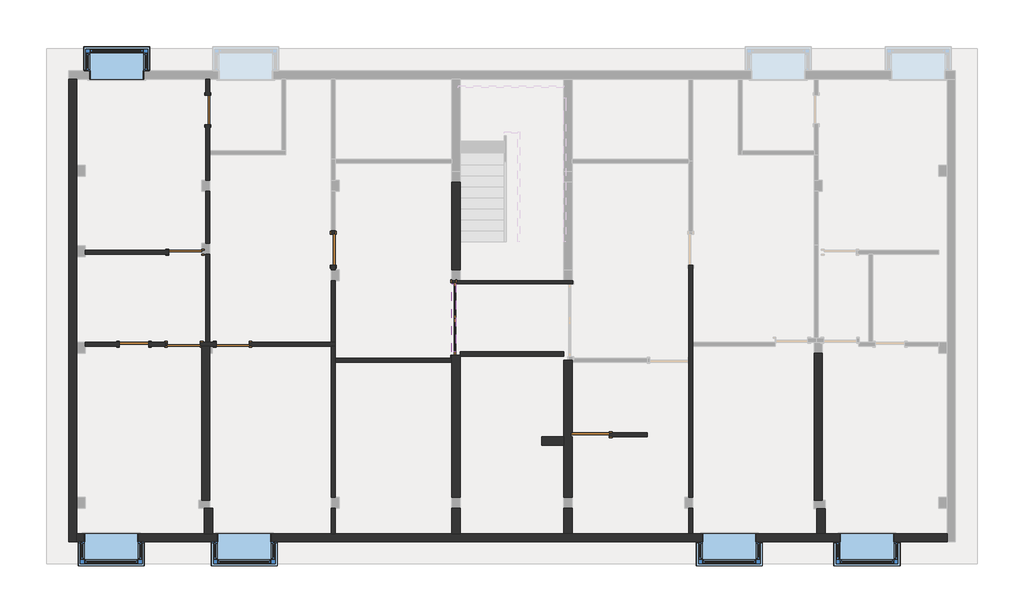
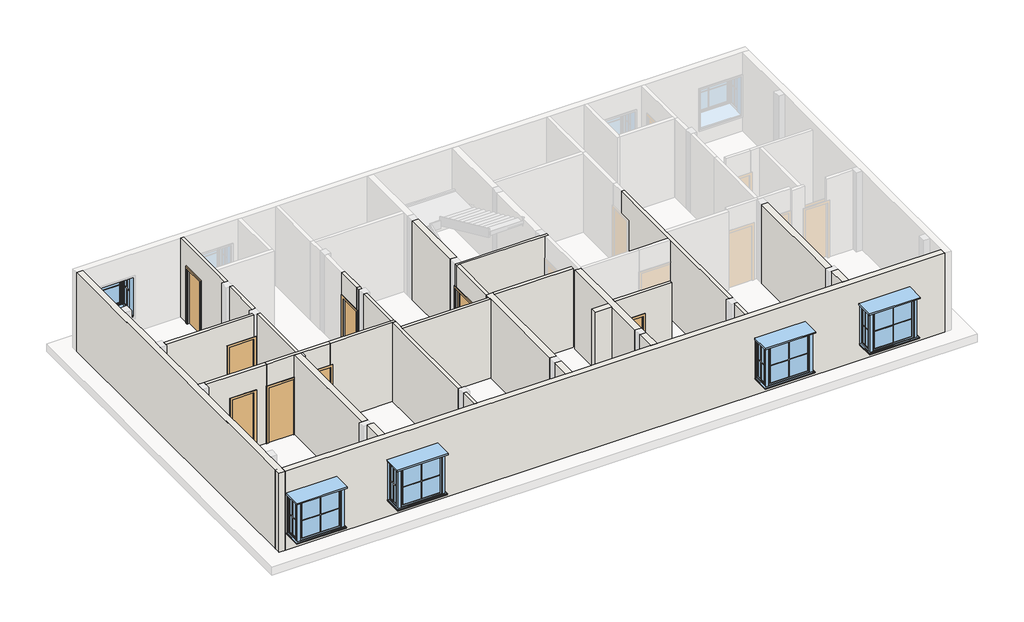
# One storey, part 1 of 3: 32 walls, 8 doors, 5 windows.
"""IFC4 building model written with IfcOpenShell, lengths in millimetres."""

from ifc_helpers import new_model, si_unit, frame, origin, place, context, project, spatial, polyline, outline, extrude, faceted_brep, transform, mapped, element, save
from components import door_04ab2522, m_door_single_panel_05506f71, door_07b5d71c, door_4c0a2014, door_82def9da, m_door_single_panel_3_x7_f8176753, m_door_single_panel_3_x7_ebb67e73, window_19bbd869

model = new_model("IFC4")

# Units and contexts
model_context = context("Model", 3, world=origin())
ifc_project = project(units=[si_unit("LENGTHUNIT", "METRE", prefix="MILLI")], contexts=[model_context])

# Site, building, storey
site = spatial("IfcSite", under=ifc_project)
building = spatial("IfcBuilding", under=site)
storey = spatial("IfcBuildingStorey", under=building, Elevation=6400.8)

# Doors
placement = place(None, origin())
door_shape = door_04ab2522(model_context)
element("IfcDoor", 1, ObjectType="M_Door-Double-Glass : 6'7\"X7'", at=placement, inside=storey, context=model_context, shape_type="MappedRepresentation", body=[
    mapped(door_shape, transform((-2022.6300498, 1231.0067742, 6400.8), x_axis=(0.0, -1.0, 0.0), y_axis=(1.0, 0.0, 0.0), z_axis=(0.0, 0.0, 1.0))),
])
m_door_single_panel_shape = m_door_single_panel_05506f71(model_context)
element("IfcDoor", 2, ObjectType="M_Door-Single-Panel", at=placement, inside=storey, context=model_context, shape_type="MappedRepresentation", body=[
    mapped(m_door_single_panel_shape, transform((1745.3012085, -1975.7432663, 6400.8), x_axis=(-1.0, 0.0, 0.0), y_axis=(0.0, -1.0, 0.0), z_axis=(0.0, 0.0, 1.0))),
])
door_2_shape = door_07b5d71c(model_context)
element("IfcDoor", 3, ObjectType="M_Door-Single-Panel : 2'10\"X7' 2", at=placement, inside=storey, context=model_context, shape_type="MappedRepresentation", body=[
    mapped(door_2_shape, transform((-5360.3487995, 3142.9626891, 6400.8), x_axis=(0.0, -1.0, 0.0), y_axis=(1.0, 0.0, 0.0), z_axis=(0.0, 0.0, 1.0))),
])
door_3_shape = door_4c0a2014(model_context)
element("IfcDoor", 4, ObjectType="M_Door-Single-Panel : 2'8\"X7'", at=placement, inside=storey, context=model_context, shape_type="MappedRepresentation", body=[
    mapped(door_3_shape, transform((-10873.4462614, 526.1567334, 6400.8), x_axis=(1.0, 0.0, 0.0), y_axis=(0.0, 1.0, 0.0), z_axis=(0.0, 0.0, 1.0))),
])
door_4_shape = door_82def9da(model_context)
element("IfcDoor", 5, ObjectType="M_Door-Single-Panel : 2'8\"X7'", at=placement, inside=storey, context=model_context, shape_type="MappedRepresentation", body=[
    mapped(door_4_shape, transform((-8827.4487992, 7008.6751452, 6400.8), x_axis=(0.0, 1.0, 0.0), y_axis=(-1.0, 0.0, 0.0), z_axis=(0.0, 0.0, 1.0))),
])
m_door_single_panel_3_x7_shape = m_door_single_panel_3_x7_f8176753(model_context)
element("IfcDoor", 6, ObjectType="M_Door-Single-Panel : 3'X7'", at=placement, inside=storey, context=model_context, shape_type="MappedRepresentation", body=[
    mapped(m_door_single_panel_3_x7_shape, transform((-9456.0987989, 3078.8567332, 6400.8), x_axis=(1.0, 0.0, 0.0), y_axis=(0.0, 1.0, 0.0), z_axis=(0.0, 0.0, 1.0))),
])
element("IfcDoor", 7, ObjectType="M_Door-Single-Panel : 3'X7'", at=placement, inside=storey, context=model_context, shape_type="MappedRepresentation", body=[
    mapped(m_door_single_panel_3_x7_shape, transform((-8144.8381465, 526.1567334, 6400.8), x_axis=(-1.0, 0.0, 0.0), y_axis=(0.0, -1.0, 0.0), z_axis=(0.0, 0.0, 1.0))),
])
m_door_single_panel_3_x7_2_shape = m_door_single_panel_3_x7_ebb67e73(model_context)
element("IfcDoor", 8, ObjectType="M_Door-Single-Panel : 3'X7'", at=placement, inside=storey, context=model_context, shape_type="MappedRepresentation", body=[
    mapped(m_door_single_panel_3_x7_2_shape, transform((-9494.1987992, 526.1567334, 6400.8), x_axis=(1.0, 0.0, 0.0), y_axis=(0.0, 1.0, 0.0), z_axis=(0.0, 0.0, 1.0))),
])

# Walls
element("IfcWall", 9, ObjectType="3.5\"", at=placement, inside=storey, context=model_context, shape_type="Brep", body=[
    faceted_brep([(1272.3082462, 2196.2067742, 9448.8), (1158.0082462, 2196.2067742, 9448.8), (-1963.0987998, 2196.2067742, 9448.8), (-2077.3987998, 2196.2067742, 9448.8), (-2077.3987998, 2196.2067742, 8534.4), (-1963.0987998, 2196.2067742, 8534.4), (-1963.0987998, 2196.2067742, 6400.8), (1158.0082462, 2196.2067742, 6400.8), (1272.3082462, 2196.2067742, 6400.8), (1272.3082462, 2285.1067742, 6400.8), (1253.2582462, 2285.1067742, 6400.8), (1024.6582462, 2285.1067742, 6400.8), (-1845.5417538, 2285.1067742, 6400.8), (-2074.1417538, 2285.1067742, 6400.8), (-2077.3987998, 2285.1067742, 6400.8), (-2077.3987998, 2285.1067742, 9448.8), (-2074.1417538, 2285.1067742, 9448.8), (-1845.5417538, 2285.1067742, 9448.8), (1024.6582462, 2285.1067742, 9448.8), (1253.2582462, 2285.1067742, 9448.8), (1272.3082462, 2285.1067742, 9448.8), (-1963.0987998, 2234.3067742, 6400.8), (-2077.3987998, 2234.3067742, 6400.8), (-2077.3987998, 2234.3067742, 8534.4), (-1963.0987998, 2234.3067742, 8534.4)], [[[0, 1, 2, 3, 4, 5, 6, 7, 8]], [[9, 10, 11, 12, 13, 14, 15, 16, 17, 18, 19, 20]], [[14, 13, 12, 11, 10, 9, 8, 7, 6, 21, 22]], [[3, 2, 1, 0, 20, 19, 18, 17, 16, 15]], [[0, 8, 9, 20]], [[3, 15, 14, 22, 23, 4]], [[24, 21, 6, 5]], [[23, 24, 5, 4]], [[21, 24, 23, 22]]]),
])
element("IfcWall", 10, ObjectType="4.5\"", at=placement, inside=storey, context=model_context, shape_type="SweptSolid", body=[
    extrude(outline(polyline([(2711.1626891, 9448.8), (3671.8272228, 9448.8), (3671.8272228, 6400.8), (3574.7626891, 6400.8), (3574.7626891, 8534.4), (2711.1626891, 8534.4), (2711.1626891, 9448.8)])), frame((-5417.4987995, 0.0, 0.0), z_axis=(1.0, 0.0, 0.0), x_axis=(0.0, 1.0, 0.0)), (0.0, 0.0, 1.0), 114.3),
])
element("IfcWall", 11, ObjectType="4.5\"", at=placement, inside=storey, context=model_context, shape_type="Brep", body=[
    faceted_brep([(-7690.1644155, 469.0067334, 9448.8), (-8713.148796, 469.0067334, 9448.8), (-8771.750543, 469.0067334, 9448.8), (-9000.350543, 469.0067334, 9448.8), (-10009.8462614, 469.0067334, 9448.8), (-10009.8462614, 469.0067334, 6400.8), (-9951.3987992, 469.0067334, 6400.8), (-9951.3987992, 469.0067334, 8534.4), (-9036.9987992, 469.0067334, 8534.4), (-9036.9987992, 469.0067334, 6400.8), (-9000.350543, 469.0067334, 6400.8), (-8771.750543, 469.0067334, 6400.8), (-8713.148796, 469.0067334, 6400.8), (-8602.0381465, 469.0067334, 6400.8), (-8602.0381465, 469.0067334, 8534.4), (-7690.1644155, 469.0067334, 8534.4), (-10009.8462614, 583.3067334, 9448.8), (-7690.1644155, 583.3067334, 9448.8), (-7690.1644155, 583.3067334, 8534.4), (-8602.0381465, 583.3067334, 8534.4), (-8602.0381465, 583.3067334, 6400.8), (-9036.9987992, 583.3067334, 6400.8), (-9036.9987992, 583.3067334, 8534.4), (-9951.3987992, 583.3067334, 8534.4), (-9951.3987992, 583.3067334, 6400.8), (-10009.8462614, 583.3067334, 6400.8)], [[[0, 1, 2, 3, 4, 5, 6, 7, 8, 9, 10, 11, 12, 13, 14, 15]], [[16, 17, 18, 19, 20, 21, 22, 23, 24, 25]], [[5, 25, 24, 6]], [[9, 21, 20, 13, 12, 11, 10]], [[17, 0, 15, 18]], [[4, 3, 2, 1, 0, 17, 16]], [[5, 4, 16, 25]], [[8, 22, 21, 9]], [[7, 23, 22, 8]], [[23, 7, 6, 24]], [[19, 14, 13, 20]], [[14, 19, 18, 15]]]),
])
element("IfcWall", 12, ObjectType="4.5\"", at=placement, inside=storey, context=model_context, shape_type="SweptSolid", body=[
    extrude(outline(polyline([(6400.8, 3334.0114184), (9448.8, 3334.0114184), (9448.8, 1250.0012085), (8534.4, 1250.0012085), (8534.4, 2278.7012085), (6400.8, 2278.7012085), (6400.8, 3334.0114184)])), frame((0.0, -2032.8932663, 0.0), z_axis=(0.0, 1.0, 0.0), x_axis=(0.0, 0.0, 1.0)), (0.0, 0.0, 1.0), 114.3),
])
element("IfcWall", 13, ObjectType="4.5\"", at=placement, inside=storey, context=model_context, shape_type="Brep", body=[
    faceted_brep([(-1848.7987998, 202.3067742, 6400.8), (1021.4012085, 202.3067742, 6400.8), (1021.4012085, 202.3067742, 9448.8), (-1848.7987998, 202.3067742, 9448.8), (-1848.7987998, 316.6067742, 6400.8), (-1848.7987998, 316.6067742, 8534.4), (-1848.7987998, 316.6067742, 9448.8), (1021.4012085, 316.6067742, 9448.8), (1021.4012085, 316.6067742, 6400.8), (-1848.7987998, 227.7067742, 6400.8)], [[[0, 1, 2, 3]], [[4, 5, 6, 7, 8]], [[1, 0, 9, 4, 8]], [[2, 1, 8, 7]], [[3, 2, 7, 6]], [[0, 3, 6, 5, 4, 9]]]),
])
element("IfcWall", 14, ObjectType="4.5\"", at=placement, inside=storey, context=model_context, shape_type="Brep", body=[
    faceted_brep([(-5417.4987995, 469.0067334, 6400.8), (-5417.4987995, -3709.2932193, 6400.8), (-5417.4987995, -3709.2932193, 9448.8), (-5417.4987995, 469.0067334, 9448.8), (-5303.1987995, 469.0067334, 6400.8), (-5303.1987995, 469.0067334, 9448.8), (-5303.1987995, 148.1078621, 9448.8), (-5303.1987995, 33.8078621, 9448.8), (-5303.1987995, -3709.2932193, 9448.8), (-5303.1987995, -3709.2932193, 6400.8), (-5303.1987995, 33.8078621, 6400.8), (-5303.1987995, 148.1078621, 6400.8)], [[[0, 1, 2, 3]], [[4, 5, 6, 7, 8, 9, 10, 11]], [[1, 0, 4, 11, 10, 9]], [[2, 1, 9, 8]], [[3, 2, 8, 7, 6, 5]], [[0, 3, 5, 4]]]),
])
element("IfcWall", 15, ObjectType="4.5\"", at=placement, inside=storey, context=model_context, shape_type="SweptSolid", body=[
    extrude(outline(polyline([(-5417.4987963, -4712.5932661), (-5417.4987963, -4014.0932193), (-5303.1987963, -4014.0932193), (-5303.1987963, -4712.5932661), (-5417.4987963, -4712.5932661)])), frame((0.0, 0.0, 6400.8), z_axis=(0.0, 0.0, 1.0), x_axis=(1.0, 0.0, 0.0)), (0.0, 0.0, 1.0), 3048.0),
])
element("IfcWall", 16, ObjectType="4.5\"", at=placement, inside=storey, context=model_context, shape_type="SweptSolid", body=[
    extrude(outline(polyline([(-1963.0987998, 2196.2067742), (-1963.0987998, 316.6067742), (-2077.3987998, 316.6067742), (-2077.3987998, 2196.2067742), (-1963.0987998, 2196.2067742)])), frame((0.0, 0.0, 8534.4), z_axis=(0.0, 0.0, 1.0), x_axis=(1.0, 0.0, 0.0)), (0.0, 0.0, 1.0), 914.4),
])
element("IfcWall", 17, ObjectType="4.5\"", at=placement, inside=storey, context=model_context, shape_type="SweptSolid", body=[
    extrude(outline(polyline([(4475.8012082, -4712.5932661), (4475.8012082, -4014.0932193), (4590.1012082, -4014.0932193), (4590.1012082, -4712.5932661), (4475.8012082, -4712.5932661)])), frame((0.0, 0.0, 6400.8), z_axis=(0.0, 0.0, 1.0), x_axis=(1.0, 0.0, 0.0)), (0.0, 0.0, 1.0), 3048.0),
])
element("IfcWall", 18, ObjectType="4.5\" 2", at=placement, inside=storey, context=model_context, shape_type="SweptSolid", body=[
    extrude(outline(polyline([(9448.8, -8998.8987989), (9448.8, -12224.6987989), (6400.8, -12224.6987989), (6400.8, -9913.2987989), (8534.4, -9913.2987989), (8534.4, -8998.8987989), (9448.8, -8998.8987989)])), frame((0.0, 3021.7067332, 0.0), z_axis=(0.0, 1.0, 0.0), x_axis=(0.0, 0.0, 1.0)), (0.0, 0.0, 1.0), 114.3),
])
element("IfcWall", 19, ObjectType="4.5\" 2", at=placement, inside=storey, context=model_context, shape_type="SweptSolid", body=[
    extrude(outline(polyline([(-8770.2987992, 4761.606733), (-8770.2987992, 3326.5067332), (-8884.5987992, 3326.5067332), (-8884.5987992, 4761.606733), (-8770.2987992, 4761.606733)])), frame((0.0, 0.0, 6400.8), z_axis=(0.0, 0.0, 1.0), x_axis=(1.0, 0.0, 0.0)), (0.0, 0.0, 1.0), 3048.0),
])
element("IfcWall", 20, ObjectType="4.5\" 2", at=placement, inside=storey, context=model_context, shape_type="Brep", body=[
    faceted_brep([(-8770.2987992, 7415.0751452, 8534.4), (-8770.2987992, 7415.0751452, 6400.8), (-8770.2987992, 7860.4067329, 6400.8), (-8770.2987992, 7860.4067329, 9448.8), (-8770.2987992, 5879.2067329, 9448.8), (-8770.2987992, 5764.9067329, 9448.8), (-8770.2987992, 5066.406733, 9448.8), (-8770.2987992, 5066.406733, 6400.8), (-8770.2987992, 5764.9067329, 6400.8), (-8770.2987992, 5879.2067329, 6400.8), (-8770.2987992, 6602.2751452, 6400.8), (-8770.2987992, 6602.2751452, 8534.4), (-8884.5987992, 7860.4067329, 6400.8), (-8884.5987992, 7415.0751452, 6400.8), (-8884.5987992, 7415.0751452, 8534.4), (-8884.5987992, 6602.2751452, 8534.4), (-8884.5987992, 6602.2751452, 6400.8), (-8884.5987992, 5066.406733, 6400.8), (-8884.5987992, 5066.406733, 9448.8), (-8884.5987992, 7860.4067329, 9448.8)], [[[0, 1, 2, 3, 4, 5, 6, 7, 8, 9, 10, 11]], [[12, 13, 14, 15, 16, 17, 18, 19]], [[2, 1, 13, 12]], [[10, 9, 8, 7, 17, 16]], [[6, 5, 4, 3, 19, 18]], [[7, 6, 18, 17]], [[14, 13, 1, 0]], [[15, 14, 0, 11]], [[16, 15, 11, 10]], [[3, 2, 12, 19]]]),
])
element("IfcWall", 21, ObjectType="4.5\" 2", at=placement, inside=storey, context=model_context, shape_type="SweptSolid", body=[
    extrude(outline(polyline([(8534.4, -10467.0462614), (6400.8, -10467.0462614), (6400.8, -10009.8462614), (9448.8, -10009.8462614), (9448.8, -12224.6987989), (6400.8, -12224.6987989), (6400.8, -11279.8462614), (8534.4, -11279.8462614), (8534.4, -10467.0462614)])), frame((0.0, 469.0067334, 0.0), z_axis=(0.0, 1.0, 0.0), x_axis=(0.0, 0.0, 1.0)), (0.0, 0.0, 1.0), 114.3),
])
element("IfcWall", 22, ObjectType="4.5\" 2", at=placement, inside=storey, context=model_context, shape_type="SweptSolid", body=[
    extrude(outline(polyline([(-8770.298796, 3021.7067332), (-8770.298796, 583.3067804), (-8884.598796, 583.3067804), (-8884.598796, 3021.7067332), (-8770.298796, 3021.7067332)])), frame((0.0, 0.0, 6400.8), z_axis=(0.0, 0.0, 1.0), x_axis=(1.0, 0.0, 0.0)), (0.0, 0.0, 1.0), 3048.0),
])
element("IfcWall", 23, ObjectType="4.5\" 2", at=placement, inside=storey, context=model_context, shape_type="Brep", body=[
    faceted_brep([(-5303.1987995, 469.0067334, 9448.8), (-5417.4987995, 469.0067334, 9448.8), (-7690.1644155, 469.0067334, 9448.8), (-7690.1644155, 469.0067334, 8534.4), (-7687.6381465, 469.0067334, 8534.4), (-7687.6381465, 469.0067334, 6400.8), (-5417.4987995, 469.0067334, 6400.8), (-5303.1987995, 469.0067334, 6400.8), (-7690.1644155, 583.3067334, 9448.8), (-5417.4987995, 583.3067334, 9448.8), (-5303.1987995, 583.3067334, 9448.8), (-5303.1987995, 583.3067334, 6400.8), (-5417.4987995, 583.3067334, 6400.8), (-7687.6381465, 583.3067334, 6400.8), (-7687.6381465, 583.3067334, 8534.4), (-7690.1644155, 583.3067334, 8534.4)], [[[0, 1, 2, 3, 4, 5, 6, 7]], [[8, 9, 10, 11, 12, 13, 14, 15]], [[11, 7, 6, 5, 13, 12]], [[2, 1, 0, 10, 9, 8]], [[2, 8, 15, 3]], [[0, 7, 11, 10]], [[14, 4, 3, 15]], [[4, 14, 13, 5]]]),
])
element("IfcWall", 24, ObjectType="4.5\" 2", at=placement, inside=storey, context=model_context, shape_type="SweptSolid", body=[
    extrude(outline(polyline([(-5303.1987995, 2285.1067802), (-5303.1987995, 583.3067334), (-5417.4987995, 583.3067334), (-5417.4987995, 2285.1067802), (-5303.1987995, 2285.1067802)])), frame((0.0, 0.0, 6400.8), z_axis=(0.0, 0.0, 1.0), x_axis=(1.0, 0.0, 0.0)), (0.0, 0.0, 1.0), 3048.0),
])
element("IfcWall", 25, ObjectType="4.5\" 2", at=placement, inside=storey, context=model_context, shape_type="Brep", body=[
    faceted_brep([(-5303.1987995, 2589.9067802, 6400.8), (-5303.1987995, 2711.1626891, 6400.8), (-5303.1987995, 2711.1626891, 8534.4), (-5303.1987995, 2711.1626891, 9448.8), (-5303.1987995, 2589.9067802, 9448.8), (-5417.4987995, 2589.9067802, 6400.8), (-5417.4987995, 2589.9067802, 9448.8), (-5417.4987995, 2711.1626891, 9448.8), (-5417.4987995, 2711.1626891, 8534.4), (-5417.4987995, 2711.1626891, 6400.8)], [[[0, 1, 2, 3, 4]], [[5, 6, 7, 8, 9]], [[1, 0, 5, 9]], [[3, 2, 1, 9, 8, 7]], [[4, 3, 7, 6]], [[0, 4, 6, 5]]]),
])
element("IfcWall", 26, ObjectType="4.5\" 2", at=placement, inside=storey, context=model_context, shape_type="Brep", body=[
    faceted_brep([(4475.8012082, -3709.2932193, 6400.8), (4475.8012082, -3709.2932193, 9448.8), (4475.8012082, 33.8078621, 9448.8), (4475.8012082, 148.1078621, 9448.8), (4475.8012082, 3132.0737955, 9448.8), (4475.8012082, 3132.0737955, 8534.4), (4475.8012082, 2711.1626891, 8534.4), (4475.8012082, 2711.1626891, 6400.8), (4475.8012082, 148.1078621, 6400.8), (4475.8012082, 33.8078621, 6400.8), (4590.1012082, -3709.2932193, 9448.8), (4590.1012082, -3709.2932193, 6400.8), (4590.1012082, 469.0067334, 6400.8), (4590.1012082, 583.3067334, 6400.8), (4590.1012082, 2711.1626891, 6400.8), (4590.1012082, 2711.1626891, 8534.4), (4590.1012082, 3132.0737955, 8534.4), (4590.1012082, 3132.0737955, 9448.8), (4590.1012082, 583.3067334, 9448.8), (4590.1012082, 469.0067334, 9448.8)], [[[0, 1, 2, 3, 4, 5, 6, 7, 8, 9]], [[10, 11, 12, 13, 14, 15, 16, 17, 18, 19]], [[11, 0, 9, 8, 7, 14, 13, 12]], [[1, 0, 11, 10]], [[4, 3, 2, 1, 10, 19, 18, 17]], [[4, 17, 16, 5]], [[6, 15, 14, 7]], [[15, 6, 5, 16]]]),
])
element("IfcWall", 27, ObjectType="4.5\" 2", at=placement, inside=storey, context=model_context, shape_type="SweptSolid", body=[
    extrude(outline(polyline([(-2077.3987998, 33.8078621), (-5303.1987995, 33.8078621), (-5303.1987995, 148.1078621), (-2077.3987998, 148.1078621), (-2077.3987998, 33.8078621)])), frame((0.0, 0.0, 6400.8), z_axis=(0.0, 0.0, 1.0), x_axis=(1.0, 0.0, 0.0)), (0.0, 0.0, 1.0), 3048.0),
])
element("IfcWall", 28, ObjectType="9\"", at=placement, inside=storey, context=model_context, shape_type="Brep", body=[
    faceted_brep([(-12453.2987957, -4941.1932661, 6400.8), (-12453.2987957, -4712.5932661, 6400.8), (-12453.2987957, -4014.0932671, 6400.8), (-12453.2987957, -3709.2932671, 6400.8), (-12453.2987957, 278.5067334, 6400.8), (-12453.2987957, 583.3067334, 6400.8), (-12453.2987957, 2951.8567332, 6400.8), (-12453.2987957, 3256.6567332, 6400.8), (-12453.2987957, 5174.3567339, 6400.8), (-12453.2987957, 5479.1567339, 6400.8), (-12453.2987957, 7860.4067329, 6400.8), (-12453.2987957, 7860.4067329, 9448.8), (-12453.2987957, 5479.1567339, 9448.8), (-12453.2987957, 5174.3567339, 9448.8), (-12453.2987957, 3256.6567332, 9448.8), (-12453.2987957, 2951.8567332, 9448.8), (-12453.2987957, 583.3067334, 9448.8), (-12453.2987957, 278.5067334, 9448.8), (-12453.2987957, -3709.2932671, 9448.8), (-12453.2987957, -4014.0932671, 9448.8), (-12453.2987957, -4712.5932661, 9448.8), (-12453.2987957, -4941.1932661, 9448.8), (-12681.8987957, -4941.1932661, 6400.8), (-12681.8987957, -4941.1932661, 9448.8), (-12681.8987957, 7860.4067329, 9448.8), (-12681.8987957, 7860.4067329, 6400.8)], [[[0, 1, 2, 3, 4, 5, 6, 7, 8, 9, 10, 11, 12, 13, 14, 15, 16, 17, 18, 19, 20, 21]], [[22, 23, 24, 25]], [[10, 9, 8, 7, 6, 5, 4, 3, 2, 1, 0, 22, 25]], [[21, 20, 19, 18, 17, 16, 15, 14, 13, 12, 11, 24, 23]], [[11, 10, 25, 24]], [[0, 21, 23, 22]]]),
])
element("IfcWall", 29, ObjectType="9\"", at=placement, inside=storey, context=model_context, shape_type="Brep", body=[
    faceted_brep([(-12453.2987957, -4712.5932661, 6400.8), (-12453.2987957, -4014.0932671, 6400.8), (-12453.2987957, -3709.2932671, 6400.8), (-12453.2987957, 278.5067334, 6400.8), (-12453.2987957, 583.3067334, 6400.8), (-12453.2987957, 2951.8567332, 6400.8), (-12453.2987957, 3256.6567332, 6400.8), (-12453.2987957, 5174.3567339, 6400.8), (-12453.2987957, 5479.1567339, 6400.8), (-12453.2987957, 7860.4067329, 6400.8), (-12453.2987957, 7860.4067329, 9448.8), (-12453.2987957, 5479.1567339, 9448.8), (-12453.2987957, 5174.3567339, 9448.8), (-12453.2987957, 3256.6567332, 9448.8), (-12453.2987957, 2951.8567332, 9448.8), (-12453.2987957, 583.3067334, 9448.8), (-12453.2987957, 278.5067334, 9448.8), (-12453.2987957, -3709.2932671, 9448.8), (-12453.2987957, -4014.0932671, 9448.8), (-12453.2987957, -4712.5932661, 9448.8), (-12681.8987957, -4712.5932661, 6400.8), (-12681.8987957, -4712.5932661, 9448.8), (-12681.8987957, 7860.4067329, 9448.8), (-12681.8987957, 7860.4067329, 6400.8)], [[[0, 1, 2, 3, 4, 5, 6, 7, 8, 9, 10, 11, 12, 13, 14, 15, 16, 17, 18, 19]], [[20, 21, 22, 23]], [[9, 8, 7, 6, 5, 4, 3, 2, 1, 0, 20, 23]], [[19, 18, 17, 16, 15, 14, 13, 12, 11, 10, 22, 21]], [[10, 9, 23, 22]], [[0, 19, 21, 20]]]),
])
element("IfcWall", 30, ObjectType="9\"", at=placement, inside=storey, context=model_context, shape_type="Brep", body=[
    faceted_brep([(-9000.350543, 469.0067334, 6400.8), (-9000.350543, -3785.4932196, 6400.8), (-9000.350543, -3785.4932196, 9448.8), (-9000.350543, 469.0067334, 9448.8), (-8771.750543, 469.0067334, 6400.8), (-8771.750543, 469.0067334, 9448.8), (-8771.750543, 278.5067334, 9448.8), (-8771.750543, -3785.4932196, 9448.8), (-8771.750543, -3785.4932196, 6400.8), (-8771.750543, 278.5067334, 6400.8)], [[[0, 1, 2, 3]], [[4, 5, 6, 7, 8, 9]], [[1, 0, 4, 9, 8]], [[2, 1, 8, 7]], [[3, 2, 7, 6, 5]], [[0, 3, 5, 4]]]),
])
element("IfcWall", 31, ObjectType="9\"", at=placement, inside=storey, context=model_context, shape_type="Brep", body=[
    faceted_brep([(-2077.3987998, -3709.2932663, 6400.8), (-2077.3987998, -3709.2932663, 9448.8), (-2077.3987998, 33.8078621, 9448.8), (-2077.3987998, 148.1078621, 9448.8), (-2077.3987998, 316.6067742, 9448.8), (-2077.3987998, 316.6067742, 8534.4), (-2077.3987998, 227.7067742, 8534.4), (-2077.3987998, 227.7067742, 6400.8), (-2077.3987998, 148.1078621, 6400.8), (-2077.3987998, 33.8078621, 6400.8), (-1848.7987998, -3709.2932663, 9448.8), (-1848.7987998, -3709.2932663, 6400.8), (-1848.7987998, 202.3067742, 6400.8), (-1848.7987998, 227.7067742, 6400.8), (-1848.7987998, 227.7067742, 8534.4), (-1848.7987998, 316.6067742, 8534.4), (-1848.7987998, 316.6067742, 9448.8), (-1848.7987998, 202.3067742, 9448.8), (-1963.0987998, 316.6067742, 9448.8), (-1963.0987998, 316.6067742, 8534.4)], [[[0, 1, 2, 3, 4, 5, 6, 7, 8, 9]], [[10, 11, 12, 13, 14, 15, 16, 17]], [[11, 0, 9, 8, 7, 13, 12]], [[1, 0, 11, 10]], [[4, 3, 2, 1, 10, 17, 16, 18]], [[4, 18, 16, 15, 19, 5]], [[6, 14, 13, 7]], [[14, 6, 5, 19, 15]]]),
])
element("IfcWall", 32, ObjectType="9\"", at=placement, inside=storey, context=model_context, shape_type="SweptSolid", body=[
    extrude(outline(polyline([(1021.4012085, -2261.4932663), (412.152227, -2261.4932663), (412.152227, -2032.8932663), (1021.4012085, -2032.8932663), (1021.4012085, -2261.4932663)])), frame((0.0, 0.0, 6400.8), z_axis=(0.0, 0.0, 1.0), x_axis=(1.0, 0.0, 0.0)), (0.0, 0.0, 1.0), 3048.0),
])
element("IfcWall", 33, ObjectType="9\"", at=placement, inside=storey, context=model_context, shape_type="Brep", body=[
    faceted_brep([(1021.4012085, 90.9578621, 6400.8), (1021.4012085, -2032.8932663, 6400.8), (1021.4012085, -2261.4932663, 6400.8), (1021.4012085, -3709.2932193, 6400.8), (1021.4012085, -3709.2932193, 9448.8), (1021.4012085, -2261.4932663, 9448.8), (1021.4012085, -2032.8932663, 9448.8), (1021.4012085, 90.9578621, 9448.8), (1250.0012085, -3709.2932193, 9448.8), (1250.0012085, -3709.2932193, 6400.8), (1250.0012085, -2032.8932663, 6400.8), (1250.0012085, -2032.8932663, 8534.4), (1250.0012085, -1918.5932663, 8534.4), (1250.0012085, -1918.5932663, 6400.8), (1250.0012085, 33.8078621, 6400.8), (1250.0012085, 90.9578621, 6400.8), (1250.0012085, 90.9578621, 9448.8), (1250.0012085, 33.8078621, 9448.8), (1250.0012085, -1918.5932663, 9448.8), (1250.0012085, -2032.8932663, 9448.8), (1158.0082462, 90.9578621, 6400.8), (1211.9012085, -1918.5932663, 6400.8), (1211.9012085, -2032.8932663, 6400.8), (1158.0082462, 90.9578621, 9448.8), (1211.9012085, -1918.5932663, 8534.4), (1211.9012085, -2032.8932663, 8534.4)], [[[0, 1, 2, 3, 4, 5, 6, 7]], [[8, 9, 10, 11, 12, 13, 14, 15, 16, 17, 18, 19]], [[3, 2, 1, 0, 20, 15, 14, 13, 21, 22, 10, 9]], [[4, 3, 9, 8]], [[7, 6, 5, 4, 8, 19, 18, 17, 16, 23]], [[0, 7, 23, 16, 15, 20]], [[24, 21, 13, 12]], [[22, 25, 11, 10]], [[21, 24, 25, 22]], [[25, 24, 12, 11]]]),
])
element("IfcWall", 34, ObjectType="9\"", at=placement, inside=storey, context=model_context, shape_type="SweptSolid", body=[
    extrude(outline(polyline([(-2074.1417538, 2589.906774), (-2074.1417538, 5015.606774), (-1845.5417538, 5015.606774), (-1845.5417538, 2589.906774), (-2074.1417538, 2589.906774)])), frame((0.0, 0.0, 6400.8), z_axis=(0.0, 0.0, 1.0), x_axis=(1.0, 0.0, 0.0)), (0.0, 0.0, 1.0), 3048.0),
])
element("IfcWall", 35, ObjectType="9\"", at=placement, inside=storey, context=model_context, shape_type="SweptSolid", body=[
    extrude(outline(polyline([(7942.9012047, -3785.4932666), (7942.9012047, 278.5067334), (8171.5012047, 278.5067334), (8171.5012047, -3785.4932666), (7942.9012047, -3785.4932666)])), frame((0.0, 0.0, 6400.8), z_axis=(0.0, 0.0, 1.0), x_axis=(1.0, 0.0, 0.0)), (0.0, 0.0, 1.0), 3048.0),
])
element("IfcWall", 36, ObjectType="9\"", at=placement, inside=storey, context=model_context, shape_type="SweptSolid", body=[
    extrude(outline(polyline([(-2077.3987998, -4712.5932661), (-2077.3987998, -4014.0932663), (-1848.7987998, -4014.0932663), (-1848.7987998, -4712.5932661), (-2077.3987998, -4712.5932661)])), frame((0.0, 0.0, 6400.8), z_axis=(0.0, 0.0, 1.0), x_axis=(1.0, 0.0, 0.0)), (0.0, 0.0, 1.0), 3048.0),
])
element("IfcWall", 37, ObjectType="9\" 2", at=placement, inside=storey, context=model_context, shape_type="Brep", body=[
    faceted_brep([(-12453.2987957, -4941.1932661, 6400.8), (11625.9012075, -4941.1932662, 6400.8), (11625.9012075, -4941.1932662, 9448.8), (-12453.2987957, -4941.1932661, 9448.8), (8658.6146942, -4941.1932661, 8551.6), (10158.6146942, -4941.1932661, 8551.6), (10158.6146942, -4941.1932661, 7000.8), (8658.6146942, -4941.1932661, 7000.8), (4849.7512082, -4941.1932661, 8551.6), (6349.7512082, -4941.1932661, 8551.6), (6349.7512082, -4941.1932661, 7000.8), (4849.7512082, -4941.1932661, 7000.8), (-8569.250543, -4941.1932661, 8551.6), (-7069.250543, -4941.1932661, 8551.6), (-7069.250543, -4941.1932661, 7000.8), (-8569.250543, -4941.1932661, 7000.8), (-12250.7987957, -4941.1932661, 8551.6), (-10750.7987957, -4941.1932661, 8551.6), (-10750.7987957, -4941.1932661, 7000.8), (-12250.7987957, -4941.1932661, 7000.8), (-12453.2987957, -4712.5932661, 6400.8), (-12453.2987957, -4712.5932661, 9448.8), (-8924.150543, -4712.5932661, 9448.8), (-8695.550543, -4712.5932661, 9448.8), (-5417.4987963, -4712.5932661, 9448.8), (-5303.1987963, -4712.5932661, 9448.8), (-2077.3987998, -4712.5932661, 9448.8), (-1848.7987998, -4712.5932661, 9448.8), (1021.4012085, -4712.5932661, 9448.8), (1250.0012085, -4712.5932661, 9448.8), (4475.8012082, -4712.5932661, 9448.8), (4590.1012082, -4712.5932661, 9448.8), (8017.9646942, -4712.5932661, 9448.8), (8246.5646942, -4712.5932661, 9448.8), (11625.9012075, -4712.5932662, 9448.8), (11625.9012075, -4712.5932662, 6400.8), (8246.5646942, -4712.5932661, 6400.8), (8017.9646942, -4712.5932661, 6400.8), (4590.1012082, -4712.5932661, 6400.8), (4475.8012082, -4712.5932661, 6400.8), (1250.0012085, -4712.5932661, 6400.8), (1021.4012085, -4712.5932661, 6400.8), (-1848.7987998, -4712.5932661, 6400.8), (-2077.3987998, -4712.5932661, 6400.8), (-5303.1987963, -4712.5932661, 6400.8), (-5417.4987963, -4712.5932661, 6400.8), (-8695.550543, -4712.5932661, 6400.8), (-8924.150543, -4712.5932661, 6400.8), (8658.6146942, -4712.5932661, 8551.6), (8658.6146942, -4712.5932661, 7000.8), (10158.6146942, -4712.5932661, 7000.8), (10158.6146942, -4712.5932661, 8551.6), (4849.7512082, -4712.5932661, 8551.6), (4849.7512082, -4712.5932661, 7000.8), (6349.7512082, -4712.5932661, 7000.8), (6349.7512082, -4712.5932661, 8551.6), (-8569.250543, -4712.5932661, 8551.6), (-8569.250543, -4712.5932661, 7000.8), (-7069.250543, -4712.5932661, 7000.8), (-7069.250543, -4712.5932661, 8551.6), (-12250.7987957, -4712.5932661, 8551.6), (-12250.7987957, -4712.5932661, 7000.8), (-10750.7987957, -4712.5932661, 7000.8), (-10750.7987957, -4712.5932661, 8551.6)], [[[0, 1, 2, 3], [4, 5, 6, 7], [8, 9, 10, 11], [12, 13, 14, 15], [16, 17, 18, 19]], [[20, 21, 22, 23, 24, 25, 26, 27, 28, 29, 30, 31, 32, 33, 34, 35, 36, 37, 38, 39, 40, 41, 42, 43, 44, 45, 46, 47], [48, 49, 50, 51], [52, 53, 54, 55], [56, 57, 58, 59], [60, 61, 62, 63]], [[1, 0, 20, 47, 46, 45, 44, 43, 42, 41, 40, 39, 38, 37, 36, 35]], [[3, 2, 34, 33, 32, 31, 30, 29, 28, 27, 26, 25, 24, 23, 22, 21]], [[2, 1, 35, 34]], [[0, 3, 21, 20]], [[49, 48, 4, 7]], [[50, 49, 7, 6]], [[51, 50, 6, 5]], [[48, 51, 5, 4]], [[53, 52, 8, 11]], [[54, 53, 11, 10]], [[55, 54, 10, 9]], [[52, 55, 9, 8]], [[57, 56, 12, 15]], [[58, 57, 15, 14]], [[59, 58, 14, 13]], [[56, 59, 13, 12]], [[61, 60, 16, 19]], [[62, 61, 19, 18]], [[63, 62, 18, 17]], [[60, 63, 17, 16]]]),
])
element("IfcWall", 38, ObjectType="9\" 2", at=placement, inside=storey, context=model_context, shape_type="Brep", body=[
    faceted_brep([(-8924.150543, -4014.0932196, 6400.8), (-8924.150543, -4712.5932661, 6400.8), (-8924.150543, -4712.5932661, 9448.8), (-8924.150543, -4014.0932196, 9448.8), (-8695.550543, -4014.0932196, 6400.8), (-8695.550543, -4014.0932196, 9448.8), (-8695.550543, -4712.5932661, 9448.8), (-8695.550543, -4712.5932661, 6400.8), (-8771.750543, -4014.0932196, 6400.8), (-8771.750543, -4014.0932196, 9448.8)], [[[0, 1, 2, 3]], [[4, 5, 6, 7]], [[1, 0, 8, 4, 7]], [[3, 2, 6, 5, 9]], [[0, 3, 9, 5, 4, 8]], [[2, 1, 7, 6]]]),
])
element("IfcWall", 39, ObjectType="9\" 2", at=placement, inside=storey, context=model_context, shape_type="SweptSolid", body=[
    extrude(outline(polyline([(1021.4012085, -4712.5932661), (1021.4012085, -4014.0932193), (1250.0012085, -4014.0932193), (1250.0012085, -4712.5932661), (1021.4012085, -4712.5932661)])), frame((0.0, 0.0, 6400.8), z_axis=(0.0, 0.0, 1.0), x_axis=(1.0, 0.0, 0.0)), (0.0, 0.0, 1.0), 3048.0),
])
element("IfcWall", 40, ObjectType="9\" 2", at=placement, inside=storey, context=model_context, shape_type="SweptSolid", body=[
    extrude(outline(polyline([(8017.9646942, -4712.5932661), (8017.9646942, -4015.9914801), (8246.5646942, -4015.9914801), (8246.5646942, -4712.5932661), (8017.9646942, -4712.5932661)])), frame((0.0, 0.0, 6400.8), z_axis=(0.0, 0.0, 1.0), x_axis=(1.0, 0.0, 0.0)), (0.0, 0.0, 1.0), 3048.0),
])

# Windows
window_shape = window_19bbd869(model_context)
element("IfcWindow", 41, ObjectType="4'.8\"x3'.8\"", at=placement, inside=storey, context=model_context, shape_type="MappedRepresentation", body=[
    mapped(window_shape, transform((-11500.7987957, -4826.8932661, 6400.8), x_axis=(-1.0, 0.0, 0.0), y_axis=(0.0, -1.0, 0.0), z_axis=(0.0, 0.0, 1.0))),
])
element("IfcWindow", 42, ObjectType="4'.8\"x3'.8\"", at=placement, inside=storey, context=model_context, shape_type="MappedRepresentation", body=[
    mapped(window_shape, transform((-7819.250543, -4826.8932661, 6400.8), x_axis=(-1.0, 0.0, 0.0), y_axis=(0.0, -1.0, 0.0), z_axis=(0.0, 0.0, 1.0))),
])
element("IfcWindow", 43, ObjectType="4'.8\"x3'.8\"", at=placement, inside=storey, context=model_context, shape_type="MappedRepresentation", body=[
    mapped(window_shape, transform((5599.7512082, -4826.8932661, 6400.8), x_axis=(-1.0, 0.0, 0.0), y_axis=(0.0, -1.0, 0.0), z_axis=(0.0, 0.0, 1.0))),
])
element("IfcWindow", 44, ObjectType="4'.8\"x3'.8\"", at=placement, inside=storey, context=model_context, shape_type="MappedRepresentation", body=[
    mapped(window_shape, transform((9408.6146942, -4826.8932661, 6400.8), x_axis=(-1.0, 0.0, 0.0), y_axis=(0.0, -1.0, 0.0), z_axis=(0.0, 0.0, 1.0))),
])
element("IfcWindow", 45, ObjectType="4'.8\"x3'.8\"", at=placement, inside=storey, context=model_context, shape_type="MappedRepresentation", body=[
    mapped(window_shape, transform((-11348.3987957, 7974.7067329, 6400.8), x_axis=(1.0, 0.0, 0.0), y_axis=(0.0, 1.0, 0.0), z_axis=(0.0, 0.0, 1.0))),
])

save(model, "model.ifc")

# Revit data of these elements
# Type "M_Door-Double-Glass : 6'7\"X7'"
#   Type Mark = "16"
#   Construction Type Id = "opn-d45"
#   Assembly Code = "C1020"
#   Analytic Construction = "Wood frame, double glass door "
#   W = 3' - 3 1/2"
#   Thickness = 0' - 1.9685"
#   Thermal Resistance (R) = 1.8150 (h·ft²·°F)/BTU
#   Swing Angle [instance default] = 90.00°
#   Heat Transfer Coefficient (U) = 0.5510 BTU/(h·ft²·°F)
#   Height = 7' - 0"
#   Bottom Rail = 0' - 3.93701"
#   Top Rail = 0' - 3.93701"
#   Stiles = 0' - 3.93701"
#   Trim Projection = 0' - 0.98425"
#   Trim Width = 0' - 3.14961"
#   Width = 6' - 7"
#   Define Thermal Properties by = 1
#   Glazing = Glass
#   Panel Material = Wood - Birch - Solid Stained Light Low Gloss
#   Trim Material = Paint - Sienna
#   Visual Light Transmittance = 0
#   Solar Heat Gain Coefficient = 0
#   Function = (empty or 0)
#   Wall Closure = (empty or 0)
# Type "M_Door-Single-Panel"
#   Type Mark = "14"
#   Construction Type Id = "DOOR"
#   Assembly Code = "C1020300"
#   Analytic Construction = "Wooden"
#   Thickness = 0' - 1.9685"
#   Thermal Resistance (R) = 2.5876 (h·ft²·°F)/BTU
#   Swing Angle [instance default] = 90.00°
#   Heat Transfer Coefficient (U) = 0.3865 BTU/(h·ft²·°F)
#   Height = 7' - 0"
#   Trim Projection Ext = 0' - 0.98425"
#   Trim Projection Int = 0' - 0.98425"
#   Trim Width = 0' - 3.14961"
#   Width = 3' - 6"
#   Define Thermal Properties by = 1
#   Panel Material = Wood - Birch - Solid Stained Light Low Gloss
#   Trim Material = Paint - Sienna
#   Visual Light Transmittance = 0
#   Solar Heat Gain Coefficient = 0
#   Function = (empty or 0)
#   Wall Closure = (empty or 0)
# Type "M_Door-Single-Panel : 2'10\"X7' 2"
#   Type Mark = "10"
#   Construction Type Id = "DOOR"
#   Assembly Code = "C1020300"
#   Analytic Construction = "Wooden"
#   Thickness = 0' - 1.9685"
#   Thermal Resistance (R) = 2.5876 (h·ft²·°F)/BTU
#   Swing Angle [instance default] = 90.00°
#   Heat Transfer Coefficient (U) = 0.3865 BTU/(h·ft²·°F)
#   Height = 7' - 0"
#   Trim Projection Ext = 0' - 0.98425"
#   Trim Projection Int = 0' - 0.98425"
#   Trim Width = 0' - 3.14961"
#   Width = 2' - 10"
#   Define Thermal Properties by = 1
#   Panel Material = Wood - Birch - Solid Stained Light Low Gloss
#   Trim Material = Paint - Sienna
#   Visual Light Transmittance = 0
#   Solar Heat Gain Coefficient = 0
#   Function = (empty or 0)
#   Wall Closure = (empty or 0)
# Type "M_Door-Single-Panel : 2'8\"X7'"
#   Type Mark = "9"
#   Construction Type Id = "DOOR"
#   Assembly Code = "C1020300"
#   Analytic Construction = "Wooden"
#   Thickness = 0' - 1.9685"
#   Thermal Resistance (R) = 2.5876 (h·ft²·°F)/BTU
#   Swing Angle [instance default] = 90.00°
#   Heat Transfer Coefficient (U) = 0.3865 BTU/(h·ft²·°F)
#   Height = 7' - 0"
#   Trim Projection Ext = 0' - 0.98425"
#   Trim Projection Int = 0' - 0.98425"
#   Trim Width = 0' - 3.14961"
#   Width = 2' - 8"
#   Define Thermal Properties by = 1
#   Panel Material = Wood - Birch - Solid Stained Light Low Gloss
#   Trim Material = Paint - Sienna
#   Visual Light Transmittance = 0
#   Solar Heat Gain Coefficient = 0
#   Function = (empty or 0)
#   Wall Closure = (empty or 0)
# Type "M_Door-Single-Panel : 3'X7'"
#   Type Mark = "11"
#   Construction Type Id = "DOOR"
#   Assembly Code = "C1020300"
#   Analytic Construction = "Wooden"
#   Thickness = 0' - 1.9685"
#   Thermal Resistance (R) = 2.5876 (h·ft²·°F)/BTU
#   Swing Angle [instance default] = 90.00°
#   Heat Transfer Coefficient (U) = 0.3865 BTU/(h·ft²·°F)
#   Height = 7' - 0"
#   Trim Projection Ext = 0' - 0.98425"
#   Trim Projection Int = 0' - 0.98425"
#   Trim Width = 0' - 3.14961"
#   Width = 3' - 0"
#   Define Thermal Properties by = 1
#   Panel Material = Wood - Birch - Solid Stained Light Low Gloss
#   Trim Material = Paint - Sienna
#   Visual Light Transmittance = 0
#   Solar Heat Gain Coefficient = 0
#   Function = (empty or 0)
#   Wall Closure = (empty or 0)
# Type "3.5\""
#   Assembly Code = "B2010"
#   Layers, outside or top first: 0' - 3 1/2" no material (function 1)
# Type "4.5\""
#   Assembly Code = "B2010"
#   Layers, outside or top first: 0' - 4 1/2" no material (function 1)
# Type "4.5\" 2"
#   Assembly Code = "B2010"
#   Layers, outside or top first: 0' - 4 1/2" no material (function 1)
# Type "9\""
#   Assembly Code = "B2010"
#   Layers, outside or top first: 0' - 9" no material (function 1)
# Type "9\" 2"
#   Assembly Code = "B2010"
#   Layers, outside or top first: 0' - 9" no material (function 1)
# Type "4'.8\"x3'.8\""
#   Type Mark = "20"
#   Fire Rating = "0.5h"
#   Assembly Code = "B2020100"
#   Analytic Construction = "1/8 in Pilkington single glazing"
#   Width = 4' - 11.05512"
#   Wall Thickness [instance default] = 0' - 5.90551"
#   Visual Light Transmittance = 0.9
#   Trim Width = 5' - 7.05512"
#   Trim Height = 4' - 11.05512"
#   Thermal Resistance (R) = 1.5394 (h·ft²·°F)/BTU
#   Solar Heat Gain Coefficient = 0.86
#   Rough Width = 4' - 11.64567"
#   Rough Height = 4' - 11.64567"
#   Height 1 = 5' - 1.05512"
#   Height = 4' - 11.05512"
#   Heat Transfer Coefficient (U) = 0.6496 BTU/(h·ft²·°F)
#   Depth = 1' - 11.62205"
#   Default Sill Height = 1' - 11.62205"
#   Side Muntin Visibility = yes
#   Center Muntin Visibility = yes
#   Interior Trim Visibility [instance default] = yes
#   Exterior Trim Visibility [instance default] = yes
#   Side Muntin Pattern = M_Muntin Pattern_2x2 : M_Muntin Pattern_2x2
#   Center Muntin Pattern = M_Muntin Pattern_2x2 : M_Muntin Pattern_2x2
#   Interior Trim Material = Wood - Stained
#   Exterior Trim Material = Clad - White
#   Exterior Trim = element 422966
#   Interior Trim = M_Trim-Window-Interior-Flat : Picture Frame
#   Interior Frame Material = Wood - Stained
#   Glass Panel Material = Glass
#   Exterior Frame Material = Clad - White
#   Wall Closure = (empty or 0)
# Element 1 (IfcDoor, "M_Door-Double-Glass : 6'7\"X7'")
#   Swing Angle = 90.00°
#   Phase Created = New Construction
#   Materials on its faces: "Wood - Birch - Solid Stained Light Low Gloss", "Paint - Sienna", "Glass"
# Element 2 (IfcDoor, "M_Door-Single-Panel")
#   Swing Angle = 90.00°
#   Phase Created = New Construction
#   Materials on its faces: "Paint - Sienna", "Wood - Birch - Solid Stained Light Low Gloss"
# Element 3 (IfcDoor, "M_Door-Single-Panel : 2'10\"X7' 2")
#   Swing Angle = 90.00°
#   Phase Created = New Construction
#   Materials on its faces: "Paint - Sienna", "Wood - Birch - Solid Stained Light Low Gloss"
# Elements 4, 5 (IfcDoor, "M_Door-Single-Panel : 2'8\"X7'")
#   Swing Angle = 90.00°
#   Phase Created = New Construction
#   Materials on its faces: "Paint - Sienna", "Wood - Birch - Solid Stained Light Low Gloss"
# Elements 6, 7, 8 (IfcDoor, "M_Door-Single-Panel : 3'X7'")
#   Swing Angle = 90.00°
#   Phase Created = New Construction
#   Materials on its faces: "Paint - Sienna", "Wood - Birch - Solid Stained Light Low Gloss"
# Element 9 (IfcWall, "3.5\"")
#   Top Offset = -0' - 6"
#   Base Offset = 0' - 0"
#   wall height = 10' - 0"
#   Phase Created = New Construction
#   Top Constraint = SECOND FLOOR
#   Materials on its faces: "Default Wall"
# Elements 10, 11, 12, 13, 14, 15, 16, 17 (IfcWall, "4.5\"")
#   Top Offset = -0' - 6"
#   Base Offset = 0' - 0"
#   wall height = 10' - 0"
#   Phase Created = New Construction
#   Top Constraint = SECOND FLOOR
#   Materials on its faces: "Default Wall"
# Elements 18, 19, 20, 21, 22, 23, 24, 25, 26, 27 (IfcWall, "4.5\" 2")
#   Top Offset = -0' - 6"
#   Base Offset = 0' - 0"
#   wall height = 10' - 0"
#   Phase Created = New Construction
#   Top Constraint = SECOND FLOOR
#   Materials on its faces: "Default Wall"
# Elements 28, 29, 30, 31, 32, 33, 34, 35, 36 (IfcWall, "9\"")
#   Top Offset = -0' - 6"
#   Base Offset = 0' - 0"
#   wall height = 10' - 0"
#   Phase Created = New Construction
#   Top Constraint = SECOND FLOOR
#   Materials on its faces: "Default Wall"
# Elements 37, 38, 39, 40 (IfcWall, "9\" 2")
#   Top Offset = -0' - 6"
#   Base Offset = 0' - 0"
#   wall height = 10' - 0"
#   Phase Created = New Construction
#   Top Constraint = SECOND FLOOR
#   Materials on its faces: "Default Wall"
# Element 41 (IfcWindow, "4'.8\"x3'.8\"")
#   Mark = "255"
#   Interior Trim Visibility = yes
#   Exterior Trim Visibility = yes
#   Phase Created = New Construction
#   Materials on its faces: "Clad - White", "Wood - Stained", "Glass"
# Element 42 (IfcWindow, "4'.8\"x3'.8\"")
#   Mark = "256"
#   Interior Trim Visibility = yes
#   Exterior Trim Visibility = yes
#   Phase Created = New Construction
#   Materials on its faces: "Clad - White", "Wood - Stained", "Glass"
# Element 43 (IfcWindow, "4'.8\"x3'.8\"")
#   Mark = "257"
#   Interior Trim Visibility = yes
#   Exterior Trim Visibility = yes
#   Phase Created = New Construction
#   Materials on its faces: "Clad - White", "Wood - Stained", "Glass"
# Element 44 (IfcWindow, "4'.8\"x3'.8\"")
#   Mark = "258"
#   Interior Trim Visibility = yes
#   Exterior Trim Visibility = yes
#   Phase Created = New Construction
#   Materials on its faces: "Clad - White", "Wood - Stained", "Glass"
# Element 45 (IfcWindow, "4'.8\"x3'.8\"")
#   Mark = "295"
#   Interior Trim Visibility = yes
#   Exterior Trim Visibility = yes
#   Phase Created = New Construction
#   Materials on its faces: "Clad - White", "Wood - Stained", "Glass"
# Materials
#   "Glass": class "Glass", colour RGB 0 128 192, transparency 0.75, Description = "Soda Lime Glass", Cost = 0
#   "Wood - Birch - Solid Stained Light Low Gloss": class "Wood", colour RGB 210 159 95, transparency 0, Cost = 0
#   "Paint - Sienna": colour RGB 118 70 51, transparency 0, Cost = 0
#   "Wood - Stained": class "Wood", colour RGB 224 178 126, transparency 0, Cost = 0
#   "Clad - White": class "Wood", colour RGB 242 242 238, transparency 0, Cost = 0
#   "Default Wall": colour RGB 128 128 128, transparency 0, Cost = 0
